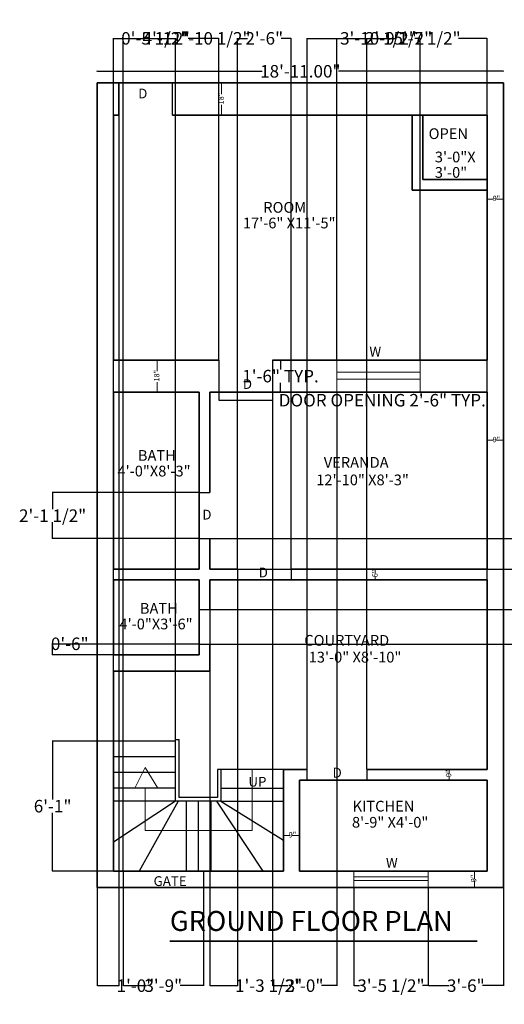
# Model space of a CAD drawing. Units: inches. Extents: x 193743 to 194406, y 400309 to 400860.
# Tile 1 of 2: x 193743 to 194014, y 400309 to 400860. Entities that reach past the tile are written whole.
import ezdxf

# ---------------------------------------------------------------- set-up
doc = ezdxf.new("R2010")
doc.units = ezdxf.units.IN
doc.header["$MEASUREMENT"] = 0
for name, color, linetype, lineweight in [('A-ANNO-DIMS', 2, 'Continuous', 18), ('A-ANNO-SYMB', 7, 'Continuous', 18), ('A-ANNO-TEXT', 7, 'Continuous', 18), ('A-ANNO-TITL', 7, 'Continuous', 35), ('A-AREA-IDEN', 7, 'Continuous', 18), ('A-DOOR', 3, 'Continuous', 25), ('A-FLOR-STRS', 7, 'Continuous', 25), ('A-GLAZ', 4, 'Continuous', 18), ('A-WALL', 7, 'Continuous', 35)]:
    doc.layers.add(name, color=color, linetype=linetype, lineweight=lineweight)
doc.styles.get("Standard").update_dxf_attribs({"font": 'arial.ttf'})
doc.dimstyles.get("Standard").update_dxf_attribs({"dimtxt": 7, "dimasz": 0.18, "dimexe": 0.18, "dimexo": 0.0625, "dimgap": 0.09, "dimtad": 0, "dimtih": 1, "dimtoh": 1, "dimzin": 0, "dimdsep": 46, "dimlunit": 3, "dimtxsty": 'Standard', "dimcen": 0.09, "dimadec": 0, "dimazin": 0, "dimtfac": 1, "dimtofl": 0, "dimtmove": 0, "dimatfit": 3, "dimfxl": 1, "dimtolj": 1, "dimtzin": 0, "dimarcsym": 0})

# ---------------------------------------------------------------- blocks, each defined once
blk = doc.blocks.new('*D1')
at = {"layer": 'A-ANNO-DIMS', "color": 0, "lineweight": -2, "transparency": 16777216}
for p, q in [((193786.7, 400830.65), (193786.7, 400830.94)), ((193786.88, 400830.76), (193878.9, 400830.76)), ((194013.52, 400830.76), (193921.5, 400830.76)), ((194013.7, 400830.65), (194013.7, 400830.94))]:
    blk.add_line(p, q, dxfattribs=at)
at = {"layer": 'A-ANNO-DIMS', "color": 0, "lineweight": 100, "transparency": 16777216}
for points in [[(193786.88, 400830.79), (193786.88, 400830.73), (193786.7, 400830.76)], [(194013.52, 400830.79), (194013.52, 400830.73), (194013.7, 400830.76)]]:
    blk.add_solid(points, dxfattribs=at)
at = {"layer": 'Defpoints', "color": 0, "lineweight": 100, "transparency": 16777216}
for p in [(193786.7, 400830.59), (194013.7, 400830.76), (194013.7, 400830.59)]:
    blk.add_point(p, dxfattribs=at)
at = {"layer": 'A-ANNO-DIMS', "color": 0, "transparency": 16777216, "insert": (193900.2, 400830.76), "char_height": 7, "attachment_point": 5}
blk.add_mtext('\\A1;18\'-11.00"', dxfattribs=at)
blk = doc.blocks.new('SHAFT-RETURN-36X36')
for p, q in [((0, 42), (0, 0)), ((6, 42), (6, 6)), ((6, 6), (42, 6)), ((0, 0), (42, 0))]:
    blk.add_line(p, q)
blk = doc.blocks.new('DOOR-OPENING-30-W18')
for p, q in [((0, 18), (0, 0)), ((29.9, 18), (29.9, 0))]:
    blk.add_line(p, q)
blk = doc.blocks.new('THICKNESS-18-V')
for p, q in [((0, 18), (0, 11.82)), ((0, 5.67), (0, 0))]:
    blk.add_line(p, q)
blk.add_text('18"', height=3, rotation=90).set_placement((1.23, 5.98))
blk = doc.blocks.new('THICKNESS-9-H')
for p, q in [((0, 1.15), (3.54, 1.15)), ((5.14, 1.15), (9, 1.15))]:
    blk.add_line(p, q)
blk.add_text('9"', height=3).set_placement((2.97, 0))
blk = doc.blocks.new('THICKNESS-9-V')
for p, q in [((0.06, 9), (0.06, 5.01)), ((0, 3.6), (0, 0))]:
    blk.add_line(p, q)
blk.add_text('9"', height=3, rotation=90).set_placement((1.05, 2.9))
blk = doc.blocks.new('ROOM-TAG-OPEN-3X3')
for s, p in [('OPEN', (0, 21.67)), ('3\'-0"X', (3.49, 8.63)), ('3\'-0"', (3.46, 0))]:
    blk.add_text(s, height=6).set_placement(p)
blk = doc.blocks.new('*D12')
at = {"layer": 'A-ANNO-DIMS', "color": 0, "lineweight": -2, "transparency": 16777216}
for p, q in [((193854.72, 400651.18), (193854.72, 400646.58)), ((193884.62, 400651.18), (193884.62, 400646.58)), ((193854.9, 400646.76), (193884.44, 400646.76)), ((193884.62, 400646.76), (193884.8, 400646.76))]:
    blk.add_line(p, q, dxfattribs=at)
at = {"layer": 'A-ANNO-DIMS', "color": 0, "lineweight": 100, "transparency": 16777216}
for points in [[(193854.9, 400646.79), (193854.9, 400646.73), (193854.72, 400646.76)], [(193884.44, 400646.79), (193884.44, 400646.73), (193884.62, 400646.76)]]:
    blk.add_solid(points, dxfattribs=at)
at = {"layer": 'Defpoints', "color": 0, "lineweight": 100, "transparency": 16777216}
for p in [(193854.72, 400651.24), (193884.62, 400651.24), (193884.62, 400646.76)]:
    blk.add_point(p, dxfattribs=at)
at = {"layer": 'A-ANNO-DIMS', "color": 0, "transparency": 16777216, "insert": (193945.99, 400646.76), "char_height": 7, "attachment_point": 5}
blk.add_mtext('\\A1;DOOR OPENING 2\'-6" TYP.', dxfattribs=at)
blk = doc.blocks.new('*D13')
at = {"layer": 'A-ANNO-DIMS', "color": 0, "lineweight": -2, "transparency": 16777216}
for p, q in [((193884.68, 400669.24), (193889.29, 400669.24)), ((193889.11, 400669.06), (193889.11, 400663.9)), ((193889.11, 400651.42), (193889.11, 400656.58)), ((193884.68, 400651.24), (193889.29, 400651.24))]:
    blk.add_line(p, q, dxfattribs=at)
at = {"layer": 'A-ANNO-DIMS', "color": 0, "lineweight": 100, "transparency": 16777216}
for points in [[(193889.08, 400669.06), (193889.14, 400669.06), (193889.11, 400669.24)], [(193889.08, 400651.42), (193889.14, 400651.42), (193889.11, 400651.24)]]:
    blk.add_solid(points, dxfattribs=at)
at = {"layer": 'Defpoints', "color": 0, "lineweight": 100, "transparency": 16777216}
for p in [(193884.62, 400669.24), (193889.11, 400669.24), (193884.62, 400651.24)]:
    blk.add_point(p, dxfattribs=at)
at = {"layer": 'A-ANNO-DIMS', "color": 0, "transparency": 16777216, "insert": (193889.11, 400660.24), "char_height": 7, "attachment_point": 5}
blk.add_mtext('\\A1;1\'-6" TYP.', dxfattribs=at)
blk = doc.blocks.new('*D18')
at = {"layer": 'A-ANNO-DIMS', "color": 0, "lineweight": -2, "transparency": 16777216}
for p, q in [((193795.7, 400383.3), (193795.7, 400849.37)), ((193795.88, 400849.19), (193800.94, 400849.19)), ((193801.12, 400383.3), (193801.12, 400849.37)), ((193801.12, 400849.19), (193801.3, 400849.19))]:
    blk.add_line(p, q, dxfattribs=at)
at = {"layer": 'A-ANNO-DIMS', "color": 0, "lineweight": 100, "transparency": 16777216}
for points in [[(193795.88, 400849.22), (193795.88, 400849.16), (193795.7, 400849.19)], [(193800.94, 400849.22), (193800.94, 400849.16), (193801.12, 400849.19)]]:
    blk.add_solid(points, dxfattribs=at)
at = {"layer": 'Defpoints', "color": 0, "lineweight": 100, "transparency": 16777216}
for p in [(193801.12, 400849.19), (193795.7, 400383.24), (193801.12, 400383.24)]:
    blk.add_point(p, dxfattribs=at)
at = {"layer": 'A-ANNO-DIMS', "color": 0, "transparency": 16777216, "insert": (193818.85, 400849.19), "char_height": 7, "attachment_point": 5}
blk.add_mtext('\\A1;0\'-5 1/2"', dxfattribs=at)
blk = doc.blocks.new('*D19')
at = {"layer": 'A-ANNO-DIMS', "color": 0, "lineweight": -2, "transparency": 16777216}
for p, q in [((193801.12, 400374.18), (193801.12, 400319.09)), ((193846.06, 400374.18), (193846.06, 400319.09)), ((193801.3, 400319.27), (193814.2, 400319.27)), ((193845.88, 400319.27), (193832.98, 400319.27))]:
    blk.add_line(p, q, dxfattribs=at)
at = {"layer": 'A-ANNO-DIMS', "color": 0, "lineweight": 100, "transparency": 16777216}
for points in [[(193801.3, 400319.3), (193801.3, 400319.24), (193801.12, 400319.27)], [(193845.88, 400319.3), (193845.88, 400319.24), (193846.06, 400319.27)]]:
    blk.add_solid(points, dxfattribs=at)
at = {"layer": 'Defpoints', "color": 0, "lineweight": 100, "transparency": 16777216}
for p in [(193801.12, 400374.24), (193846.06, 400374.24), (193846.06, 400319.27)]:
    blk.add_point(p, dxfattribs=at)
at = {"layer": 'A-ANNO-DIMS', "color": 0, "transparency": 16777216, "insert": (193823.59, 400319.27), "char_height": 7, "attachment_point": 5}
blk.add_mtext('\\A1;3\'-9"', dxfattribs=at)
blk = doc.blocks.new('*D20')
at = {"layer": 'A-ANNO-DIMS', "color": 0, "lineweight": -2, "transparency": 16777216}
for p, q in [((193930.04, 400374.18), (193930.04, 400319.09)), ((193971.71, 400374.18), (193971.71, 400319.09)), ((193930.22, 400319.27), (193933.33, 400319.27)), ((193971.53, 400319.27), (193968.42, 400319.27))]:
    blk.add_line(p, q, dxfattribs=at)
at = {"layer": 'A-ANNO-DIMS', "color": 0, "lineweight": 100, "transparency": 16777216}
for points in [[(193930.22, 400319.3), (193930.22, 400319.24), (193930.04, 400319.27)], [(193971.53, 400319.3), (193971.53, 400319.24), (193971.71, 400319.27)]]:
    blk.add_solid(points, dxfattribs=at)
at = {"layer": 'Defpoints', "color": 0, "lineweight": 100, "transparency": 16777216}
for p in [(193930.04, 400374.24), (193971.71, 400374.24), (193971.71, 400319.27)]:
    blk.add_point(p, dxfattribs=at)
at = {"layer": 'A-ANNO-DIMS', "color": 0, "transparency": 16777216, "insert": (193950.87, 400319.27), "char_height": 7, "attachment_point": 5}
blk.add_mtext('\\A1;3\'-5 1/2"', dxfattribs=at)
blk = doc.blocks.new('*D21')
at = {"layer": 'A-ANNO-DIMS', "color": 0, "lineweight": -2, "transparency": 16777216}
for p, q in [((193971.71, 400374.18), (193971.71, 400319.09)), ((194013.7, 400374.18), (194013.7, 400319.09)), ((193971.89, 400319.27), (193983.31, 400319.27)), ((194013.52, 400319.27), (194002.09, 400319.27))]:
    blk.add_line(p, q, dxfattribs=at)
at = {"layer": 'A-ANNO-DIMS', "color": 0, "lineweight": 100, "transparency": 16777216}
for points in [[(193971.89, 400319.3), (193971.89, 400319.24), (193971.71, 400319.27)], [(194013.52, 400319.3), (194013.52, 400319.24), (194013.7, 400319.27)]]:
    blk.add_solid(points, dxfattribs=at)
at = {"layer": 'Defpoints', "color": 0, "lineweight": 100, "transparency": 16777216}
for p in [(193971.71, 400374.24), (194013.7, 400374.24), (194013.7, 400319.27)]:
    blk.add_point(p, dxfattribs=at)
at = {"layer": 'A-ANNO-DIMS', "color": 0, "transparency": 16777216, "insert": (193992.7, 400319.27), "char_height": 7, "attachment_point": 5}
blk.add_mtext('\\A1;3\'-6"', dxfattribs=at)
blk = doc.blocks.new('*D22')
at = {"layer": 'A-ANNO-DIMS', "color": 0, "lineweight": -2, "transparency": 16777216}
for p, q in [((193786.7, 400824.18), (193786.7, 400319.09)), ((193798.79, 400824.18), (193798.79, 400319.09)), ((193786.88, 400319.27), (193798.61, 400319.27)), ((193798.79, 400319.27), (193798.97, 400319.27))]:
    blk.add_line(p, q, dxfattribs=at)
at = {"layer": 'A-ANNO-DIMS', "color": 0, "lineweight": 100, "transparency": 16777216}
for points in [[(193786.88, 400319.3), (193786.88, 400319.24), (193786.7, 400319.27)], [(193798.61, 400319.3), (193798.61, 400319.24), (193798.79, 400319.27)]]:
    blk.add_solid(points, dxfattribs=at)
at = {"layer": 'Defpoints', "color": 0, "lineweight": 100, "transparency": 16777216}
for p in [(193786.7, 400824.24), (193798.79, 400824.24), (193798.79, 400319.27)]:
    blk.add_point(p, dxfattribs=at)
at = {"layer": 'A-ANNO-DIMS', "color": 0, "transparency": 16777216, "insert": (193808.03, 400319.27), "char_height": 7, "attachment_point": 5}
blk.add_mtext('\\A1;1\'-0"', dxfattribs=at)
blk = doc.blocks.new('*D23')
at = {"layer": 'A-ANNO-DIMS', "color": 0, "lineweight": -2, "transparency": 16777216}
for p, q in [((193795.7, 400669.3), (193795.7, 400849.37)), ((193795.88, 400849.19), (193812.95, 400849.19)), ((193854.54, 400849.19), (193837.46, 400849.19)), ((193854.72, 400669.3), (193854.72, 400849.37))]:
    blk.add_line(p, q, dxfattribs=at)
at = {"layer": 'A-ANNO-DIMS', "color": 0, "lineweight": 100, "transparency": 16777216}
for points in [[(193795.88, 400849.22), (193795.88, 400849.16), (193795.7, 400849.19)], [(193854.54, 400849.22), (193854.54, 400849.16), (193854.72, 400849.19)]]:
    blk.add_solid(points, dxfattribs=at)
at = {"layer": 'Defpoints', "color": 0, "lineweight": 100, "transparency": 16777216}
for p in [(193854.72, 400849.19), (193795.7, 400669.24), (193854.72, 400669.24)]:
    blk.add_point(p, dxfattribs=at)
at = {"layer": 'A-ANNO-DIMS', "color": 0, "transparency": 16777216, "insert": (193825.21, 400849.19), "char_height": 7, "attachment_point": 5}
blk.add_mtext('\\A1;4\'-11"', dxfattribs=at)
blk = doc.blocks.new('*D24')
at = {"layer": 'A-ANNO-DIMS', "color": 0, "lineweight": -2, "transparency": 16777216}
for p, q in [((193920.54, 400669.3), (193920.54, 400849.37)), ((193920.72, 400849.19), (193923.58, 400849.19)), ((193966.98, 400849.19), (193964.12, 400849.19)), ((193967.16, 400669.3), (193967.16, 400849.37))]:
    blk.add_line(p, q, dxfattribs=at)
at = {"layer": 'A-ANNO-DIMS', "color": 0, "lineweight": 100, "transparency": 16777216}
for points in [[(193920.72, 400849.22), (193920.72, 400849.16), (193920.54, 400849.19)], [(193966.98, 400849.22), (193966.98, 400849.16), (193967.16, 400849.19)]]:
    blk.add_solid(points, dxfattribs=at)
at = {"layer": 'Defpoints', "color": 0, "lineweight": 100, "transparency": 16777216}
for p in [(193967.16, 400849.19), (193920.54, 400669.24), (193967.16, 400669.24)]:
    blk.add_point(p, dxfattribs=at)
at = {"layer": 'A-ANNO-DIMS', "color": 0, "transparency": 16777216, "insert": (193943.85, 400849.19), "char_height": 7, "attachment_point": 5}
blk.add_mtext('\\A1;3\'-10 1/2"', dxfattribs=at)
blk = doc.blocks.new('*D25')
at = {"layer": 'A-ANNO-DIMS', "color": 0, "lineweight": -2, "transparency": 16777216}
for p, q in [((193884.62, 400651.18), (193884.62, 400319.09)), ((193920.54, 400651.18), (193920.54, 400319.09)), ((193884.8, 400319.27), (193893.19, 400319.27)), ((193920.36, 400319.27), (193911.97, 400319.27))]:
    blk.add_line(p, q, dxfattribs=at)
at = {"layer": 'A-ANNO-DIMS', "color": 0, "lineweight": 100, "transparency": 16777216}
for points in [[(193884.8, 400319.3), (193884.8, 400319.24), (193884.62, 400319.27)], [(193920.36, 400319.3), (193920.36, 400319.24), (193920.54, 400319.27)]]:
    blk.add_solid(points, dxfattribs=at)
at = {"layer": 'Defpoints', "color": 0, "lineweight": 100, "transparency": 16777216}
for p in [(193884.62, 400651.24), (193920.54, 400651.24), (193920.54, 400319.27)]:
    blk.add_point(p, dxfattribs=at)
at = {"layer": 'A-ANNO-DIMS', "color": 0, "transparency": 16777216, "insert": (193902.58, 400319.27), "char_height": 7, "attachment_point": 5}
blk.add_mtext('\\A1;3\'-0"', dxfattribs=at)
blk = doc.blocks.new('*D26')
at = {"layer": 'A-ANNO-DIMS', "color": 0, "lineweight": -2, "transparency": 16777216}
for p, q in [((193849.7, 400546.18), (193849.7, 400319.09)), ((193865.1, 400546.18), (193865.1, 400319.09)), ((193849.88, 400319.27), (193864.92, 400319.27)), ((193865.1, 400319.27), (193865.28, 400319.27))]:
    blk.add_line(p, q, dxfattribs=at)
at = {"layer": 'A-ANNO-DIMS', "color": 0, "lineweight": 100, "transparency": 16777216}
for points in [[(193849.88, 400319.3), (193849.88, 400319.24), (193849.7, 400319.27)], [(193864.92, 400319.3), (193864.92, 400319.24), (193865.1, 400319.27)]]:
    blk.add_solid(points, dxfattribs=at)
at = {"layer": 'Defpoints', "color": 0, "lineweight": 100, "transparency": 16777216}
for p in [(193849.7, 400546.24), (193865.1, 400546.24), (193865.1, 400319.27)]:
    blk.add_point(p, dxfattribs=at)
at = {"layer": 'A-ANNO-DIMS', "color": 0, "transparency": 16777216, "insert": (193882.5, 400319.27), "char_height": 7, "attachment_point": 5}
blk.add_mtext('\\A1;1\'-3 1/2"', dxfattribs=at)
blk = doc.blocks.new('*D27')
at = {"layer": 'A-ANNO-DIMS', "color": 0, "lineweight": -2, "transparency": 16777216}
for p, q in [((193865.1, 400552.3), (193865.1, 400849.37)), ((193865.28, 400849.19), (193870.6, 400849.19)), ((193894.82, 400849.19), (193889.51, 400849.19)), ((193895, 400552.3), (193895, 400849.37))]:
    blk.add_line(p, q, dxfattribs=at)
at = {"layer": 'A-ANNO-DIMS', "color": 0, "lineweight": 100, "transparency": 16777216}
for points in [[(193865.28, 400849.22), (193865.28, 400849.16), (193865.1, 400849.19)], [(193894.82, 400849.22), (193894.82, 400849.16), (193895, 400849.19)]]:
    blk.add_solid(points, dxfattribs=at)
at = {"layer": 'Defpoints', "color": 0, "lineweight": 100, "transparency": 16777216}
for p in [(193895, 400849.19), (193865.1, 400552.24), (193895, 400552.24)]:
    blk.add_point(p, dxfattribs=at)
at = {"layer": 'A-ANNO-DIMS', "color": 0, "transparency": 16777216, "insert": (193880.05, 400849.19), "char_height": 7, "attachment_point": 5}
blk.add_mtext('\\A1;2\'-6"', dxfattribs=at)
blk = doc.blocks.new('*D28')
at = {"layer": 'A-ANNO-DIMS', "color": 0, "lineweight": -2, "transparency": 16777216}
for p, q in [((193849.76, 400569.32), (194038.83, 400569.32)), ((194038.65, 400569.14), (194038.65, 400564.44)), ((194038.65, 400552.42), (194038.65, 400557.12)), ((193849.76, 400552.24), (194038.83, 400552.24))]:
    blk.add_line(p, q, dxfattribs=at)
at = {"layer": 'A-ANNO-DIMS', "color": 0, "lineweight": 100, "transparency": 16777216}
for points in [[(194038.62, 400569.14), (194038.68, 400569.14), (194038.65, 400569.32)], [(194038.62, 400552.42), (194038.68, 400552.42), (194038.65, 400552.24)]]:
    blk.add_solid(points, dxfattribs=at)
at = {"layer": 'Defpoints', "color": 0, "lineweight": 100, "transparency": 16777216}
for p in [(193849.7, 400569.32), (194038.65, 400569.32), (193849.7, 400552.24)]:
    blk.add_point(p, dxfattribs=at)
at = {"layer": 'A-ANNO-DIMS', "color": 0, "transparency": 16777216, "insert": (194038.65, 400560.78), "char_height": 7, "attachment_point": 5}
blk.add_mtext('\\A1;1\'-5"', dxfattribs=at)
blk = doc.blocks.new('*D29')
at = {"layer": 'A-ANNO-DIMS', "color": 0, "lineweight": -2, "transparency": 16777216}
for p, q in [((193843.63, 400595.05), (193761.57, 400595.05)), ((193761.75, 400594.87), (193761.75, 400585.89)), ((193761.75, 400569.5), (193761.75, 400578.48)), ((193843.63, 400569.32), (193761.57, 400569.32))]:
    blk.add_line(p, q, dxfattribs=at)
at = {"layer": 'A-ANNO-DIMS', "color": 0, "lineweight": 100, "transparency": 16777216}
for points in [[(193761.72, 400594.87), (193761.78, 400594.87), (193761.75, 400595.05)], [(193761.72, 400569.5), (193761.78, 400569.5), (193761.75, 400569.32)]]:
    blk.add_solid(points, dxfattribs=at)
at = {"layer": 'Defpoints', "color": 0, "lineweight": 100, "transparency": 16777216}
for p in [(193761.75, 400595.05), (193843.7, 400595.05), (193843.7, 400569.32)]:
    blk.add_point(p, dxfattribs=at)
at = {"layer": 'A-ANNO-DIMS', "color": 0, "transparency": 16777216, "insert": (193761.75, 400582.19), "char_height": 7, "attachment_point": 5}
blk.add_mtext('\\A1;2\'-1 1/2"', dxfattribs=at)
blk = doc.blocks.new('*D30')
at = {"layer": 'A-ANNO-DIMS', "color": 0, "lineweight": -2, "transparency": 16777216}
for p, q in [((193843.63, 400510.32), (193761.57, 400510.32)), ((193761.75, 400510.32), (193761.75, 400510.5)), ((193761.75, 400510.5), (193761.93, 400510.5)), ((193761.75, 400504.42), (193761.75, 400510.14)), ((193843.63, 400504.24), (193761.57, 400504.24))]:
    blk.add_line(p, q, dxfattribs=at)
at = {"layer": 'A-ANNO-DIMS', "color": 0, "lineweight": 100, "transparency": 16777216}
for points in [[(193761.72, 400510.14), (193761.78, 400510.14), (193761.75, 400510.32)], [(193761.72, 400504.42), (193761.78, 400504.42), (193761.75, 400504.24)]]:
    blk.add_solid(points, dxfattribs=at)
at = {"layer": 'Defpoints', "color": 0, "lineweight": 100, "transparency": 16777216}
for p in [(193761.75, 400510.32), (193843.7, 400510.32), (193843.7, 400504.24)]:
    blk.add_point(p, dxfattribs=at)
at = {"layer": 'A-ANNO-DIMS', "color": 0, "transparency": 16777216, "insert": (193771.32, 400510.5), "char_height": 7, "attachment_point": 5}
blk.add_mtext('\\A1;0\'-6"', dxfattribs=at)
blk = doc.blocks.new('*D31')
at = {"layer": 'A-ANNO-DIMS', "color": 0, "lineweight": -2, "transparency": 16777216}
for p, q in [((193849.76, 400529.76), (194038.83, 400529.76)), ((194038.65, 400529.58), (194038.65, 400523.75)), ((194038.65, 400510.5), (194038.65, 400516.33)), ((193849.76, 400510.32), (194038.83, 400510.32))]:
    blk.add_line(p, q, dxfattribs=at)
at = {"layer": 'A-ANNO-DIMS', "color": 0, "lineweight": 100, "transparency": 16777216}
for points in [[(194038.62, 400529.58), (194038.68, 400529.58), (194038.65, 400529.76)], [(194038.62, 400510.5), (194038.68, 400510.5), (194038.65, 400510.32)]]:
    blk.add_solid(points, dxfattribs=at)
at = {"layer": 'Defpoints', "color": 0, "lineweight": 100, "transparency": 16777216}
for p in [(193849.7, 400529.76), (193849.7, 400510.32), (194038.65, 400510.32)]:
    blk.add_point(p, dxfattribs=at)
at = {"layer": 'A-ANNO-DIMS', "color": 0, "transparency": 16777216, "insert": (194038.65, 400520.04), "char_height": 7, "attachment_point": 5}
blk.add_mtext('\\A1;1\'-7 1/2"', dxfattribs=at)
blk = doc.blocks.new('*D32')
at = {"layer": 'A-ANNO-DIMS', "color": 0, "lineweight": -2, "transparency": 16777216}
for p, q in [((193904.1, 400440.3), (193904.1, 400849.37)), ((193904.28, 400849.19), (193937.18, 400849.19)), ((193937.36, 400440.3), (193937.36, 400849.37)), ((193937.36, 400849.19), (193937.54, 400849.19))]:
    blk.add_line(p, q, dxfattribs=at)
at = {"layer": 'A-ANNO-DIMS', "color": 0, "lineweight": 100, "transparency": 16777216}
for points in [[(193904.28, 400849.22), (193904.28, 400849.16), (193904.1, 400849.19)], [(193937.18, 400849.22), (193937.18, 400849.16), (193937.36, 400849.19)]]:
    blk.add_solid(points, dxfattribs=at)
at = {"layer": 'Defpoints', "color": 0, "lineweight": 100, "transparency": 16777216}
for p in [(193937.36, 400849.19), (193904.1, 400440.24), (193937.36, 400440.24)]:
    blk.add_point(p, dxfattribs=at)
at = {"layer": 'A-ANNO-DIMS', "color": 0, "transparency": 16777216, "insert": (193955.15, 400849.19), "char_height": 7, "attachment_point": 5}
blk.add_mtext('\\A1;2\'-9 1/2"', dxfattribs=at)
blk = doc.blocks.new('*D33')
at = {"layer": 'A-ANNO-DIMS', "color": 0, "lineweight": -2, "transparency": 16777216}
for p, q in [((193937.36, 400440.3), (193937.36, 400849.37)), ((193937.54, 400849.19), (193953.48, 400849.19)), ((194004.52, 400849.19), (193988.58, 400849.19)), ((194004.7, 400440.3), (194004.7, 400849.37))]:
    blk.add_line(p, q, dxfattribs=at)
at = {"layer": 'A-ANNO-DIMS', "color": 0, "lineweight": 100, "transparency": 16777216}
for points in [[(193937.54, 400849.22), (193937.54, 400849.16), (193937.36, 400849.19)], [(194004.52, 400849.22), (194004.52, 400849.16), (194004.7, 400849.19)]]:
    blk.add_solid(points, dxfattribs=at)
at = {"layer": 'Defpoints', "color": 0, "lineweight": 100, "transparency": 16777216}
for p in [(194004.7, 400849.19), (193937.36, 400440.24), (194004.7, 400440.24)]:
    blk.add_point(p, dxfattribs=at)
at = {"layer": 'A-ANNO-DIMS', "color": 0, "transparency": 16777216, "insert": (193971.03, 400849.19), "char_height": 7, "attachment_point": 5}
blk.add_mtext('\\A1;5\'-7 1/2"', dxfattribs=at)
blk = doc.blocks.new('*D34')
at = {"layer": 'A-ANNO-DIMS', "color": 0, "lineweight": -2, "transparency": 16777216}
for p, q in [((193795.7, 400456.18), (193795.7, 400849.37)), ((193795.88, 400849.19), (193830.26, 400849.19)), ((193830.44, 400456.18), (193830.44, 400849.37)), ((193830.44, 400849.19), (193830.62, 400849.19))]:
    blk.add_line(p, q, dxfattribs=at)
at = {"layer": 'A-ANNO-DIMS', "color": 0, "lineweight": 100, "transparency": 16777216}
for points in [[(193795.88, 400849.22), (193795.88, 400849.16), (193795.7, 400849.19)], [(193830.26, 400849.22), (193830.26, 400849.16), (193830.44, 400849.19)]]:
    blk.add_solid(points, dxfattribs=at)
at = {"layer": 'Defpoints', "color": 0, "lineweight": 100, "transparency": 16777216}
for p in [(193830.44, 400849.19), (193795.7, 400456.12), (193830.44, 400456.12)]:
    blk.add_point(p, dxfattribs=at)
at = {"layer": 'A-ANNO-DIMS', "color": 0, "transparency": 16777216, "insert": (193850.94, 400849.19), "char_height": 7, "attachment_point": 5}
blk.add_mtext('\\A1;2\'-10 1/2"', dxfattribs=at)
blk = doc.blocks.new('*D35')
at = {"layer": 'A-ANNO-DIMS', "color": 0, "lineweight": -2, "transparency": 16777216}
for p, q in [((193795.63, 400456.12), (193761.57, 400456.12)), ((193761.75, 400455.94), (193761.75, 400423.35)), ((193761.75, 400383.42), (193761.75, 400416.02)), ((193795.63, 400383.24), (193761.57, 400383.24))]:
    blk.add_line(p, q, dxfattribs=at)
at = {"layer": 'A-ANNO-DIMS', "color": 0, "lineweight": 100, "transparency": 16777216}
for points in [[(193761.72, 400455.94), (193761.78, 400455.94), (193761.75, 400456.12)], [(193761.72, 400383.42), (193761.78, 400383.42), (193761.75, 400383.24)]]:
    blk.add_solid(points, dxfattribs=at)
at = {"layer": 'Defpoints', "color": 0, "lineweight": 100, "transparency": 16777216}
for p in [(193761.75, 400456.12), (193795.7, 400456.12), (193795.7, 400383.24)]:
    blk.add_point(p, dxfattribs=at)
at = {"layer": 'A-ANNO-DIMS', "color": 0, "transparency": 16777216, "insert": (193761.75, 400419.68), "char_height": 7, "attachment_point": 5}
blk.add_mtext('\\A1;6\'-1"', dxfattribs=at)

msp = doc.modelspace()

# ---------------------------------------------------------------- linework, layer by layer
at = {"layer": 'A-ANNO-DIMS'}
for p, q in [((193942.101, 400552.24), (193942.101, 400552.24)), ((193942.101, 400552.24), (193942.101, 400549.774)), ((193942.101, 400547.811), (193942.101, 400546.24)), ((193983.342, 400438.066), (193983.342, 400440.24)), ((193983.342, 400436.447), (193983.342, 400434.24))]:
    msp.add_line(p, q, dxfattribs=at)
at = {"layer": 'A-ANNO-SYMB'}
for p, q in [((193807.697, 400429.723), (193813.541, 400441.344)), ((193813.541, 400441.344), (193820.557, 400429.723)), ((193873.253, 400440.24), (193873.253, 400406.096)), ((193813.541, 400429.723), (193807.697, 400429.723)), ((193813.541, 400406.096), (193813.541, 400429.723)), ((193873.253, 400406.096), (193813.541, 400406.096))]:
    msp.add_line(p, q, dxfattribs=at)
at = {"layer": 'A-ANNO-TITL'}
msp.add_line((193827.283, 400344.223), (193999.094, 400344.223), dxfattribs=at)
at = {"layer": 'A-DOOR'}
for p, q in [((193843.697, 400595.052), (193849.697, 400595.052)), ((193843.697, 400569.318), (193849.697, 400569.318)), ((193865.104, 400552.24), (193865.104, 400546.24)), ((193895.003, 400552.24), (193895.003, 400546.24)), ((193843.697, 400529.763), (193849.697, 400529.763)), ((193843.697, 400510.321), (193849.697, 400510.321)), ((193904.104, 400434.24), (193904.104, 400440.24)), ((193937.364, 400440.24), (193937.364, 400434.24)), ((193801.119, 400383.24), (193801.119, 400374.24)), ((193846.055, 400383.24), (193846.055, 400374.24))]:
    msp.add_line(p, q, dxfattribs=at)
at = {"layer": 'A-FLOR-STRS'}
for p, q in [((193830.436, 400456.122), (193795.697, 400456.122)), ((193830.436, 400422.546), (193830.436, 400457.001)), ((193830.436, 400457.001), (193832.436, 400457.001)), ((193832.436, 400424.546), (193832.436, 400457.001)), ((193830.436, 400447.322), (193795.697, 400447.322)), ((193830.436, 400438.523), (193795.697, 400438.523)), ((193890.697, 400440.24), (193853.809, 400440.24)), ((193853.809, 400440.24), (193853.809, 400424.546)), ((193855.809, 400440.24), (193855.809, 400422.546)), ((193830.436, 400429.723), (193795.697, 400429.723)), ((193855.809, 400429.723), (193890.697, 400429.723)), ((193830.436, 400422.546), (193795.697, 400422.546)), ((193830.436, 400422.546), (193795.697, 400399.547)), ((193831.952, 400422.546), (193810.193, 400383.24)), ((193855.809, 400422.546), (193830.436, 400422.546)), ((193853.809, 400424.546), (193832.436, 400424.546)), ((193836.323, 400422.546), (193836.323, 400383.24)), ((193843.123, 400422.546), (193843.123, 400383.24)), ((193850.233, 400422.546), (193850.233, 400383.24)), ((193853.412, 400422.546), (193879.244, 400383.24)), ((193855.809, 400422.546), (193890.697, 400400.738)), ((193855.809, 400422.546), (193890.697, 400422.546))]:
    msp.add_line(p, q, dxfattribs=at)
at = {"layer": 'A-GLAZ'}
for p, q in [((193920.537, 400669.24), (193920.537, 400651.24)), ((193967.161, 400669.24), (193967.161, 400669.24)), ((193967.161, 400669.24), (193967.161, 400651.24)), ((193920.537, 400662.472), (193967.161, 400662.472)), ((193920.537, 400658.511), (193967.161, 400658.511)), ((193930.039, 400383.24), (193930.039, 400374.24)), ((193971.709, 400383.24), (193971.709, 400374.24)), ((193971.709, 400380.221), (193930.039, 400380.221)), ((193930.039, 400380.221), (193930.039, 400378.07)), ((193930.039, 400378.07), (193971.709, 400378.07)), ((193971.709, 400374.24), (193971.709, 400380.221))]:
    msp.add_line(p, q, dxfattribs=at)
at = {"layer": 'A-WALL'}
for p, q in [((193786.697, 400824.24), (194013.697, 400824.24)), ((193786.697, 400374.24), (193786.697, 400824.24)), ((194013.697, 400824.24), (194013.697, 400374.24)), ((193795.697, 400806.24), (193798.787, 400806.24)), ((193795.697, 400669.24), (193795.697, 400806.24)), ((193828.686, 400806.24), (194004.697, 400806.24)), ((194004.697, 400806.24), (194004.697, 400669.24)), ((193795.697, 400669.24), (193854.721, 400669.24)), ((193884.621, 400669.24), (194004.697, 400669.24)), ((193795.697, 400651.24), (193843.697, 400651.24)), ((193795.697, 400552.24), (193795.697, 400651.24)), ((193843.697, 400552.24), (193843.697, 400651.24)), ((193843.697, 400552.24), (193843.697, 400651.24)), ((193849.697, 400651.24), (194004.697, 400651.24)), ((193849.697, 400595.052), (193849.697, 400651.24)), ((193849.697, 400595.052), (193849.697, 400651.24)), ((194004.697, 400651.24), (194004.697, 400552.24)), ((193849.697, 400552.24), (193849.697, 400569.318)), ((193849.697, 400552.24), (193849.697, 400569.318)), ((193795.697, 400552.24), (193843.697, 400552.24)), ((193849.697, 400552.24), (193865.104, 400552.24)), ((193895.003, 400552.24), (194004.697, 400552.24)), ((193795.697, 400546.24), (193843.697, 400546.24)), ((193795.697, 400504.24), (193795.697, 400546.24)), ((193843.697, 400504.24), (193843.697, 400546.24)), ((193849.697, 400546.24), (194004.697, 400546.24)), ((193849.697, 400529.763), (193849.697, 400546.24)), ((194004.697, 400546.24), (194004.697, 400440.24)), ((193849.697, 400495.24), (193849.697, 400510.321)), ((193795.697, 400504.24), (193843.697, 400504.24)), ((193795.697, 400383.24), (193795.697, 400495.24)), ((193795.697, 400495.24), (193849.697, 400495.24)), ((193890.697, 400440.24), (193904.104, 400440.24)), ((193890.697, 400440.24), (193890.697, 400383.24)), ((193937.364, 400440.24), (194004.697, 400440.24)), ((193899.697, 400434.24), (194004.697, 400434.24)), ((193899.697, 400434.24), (193899.697, 400383.24)), ((194004.697, 400434.24), (194004.697, 400383.24)), ((193890.697, 400383.24), (193795.697, 400383.24)), ((194004.697, 400383.24), (193899.697, 400383.24)), ((194013.697, 400374.24), (193786.697, 400374.24))]:
    msp.add_line(p, q, dxfattribs=at)

# ---------------------------------------------------------------- block references
at = {"layer": 'A-ANNO-DIMS'}
for name, p in [('THICKNESS-18-V', (193856.126, 400806.24)), ('THICKNESS-9-H', (194004.697, 400758.15)), ('THICKNESS-18-V', (193820.16, 400651.24)), ('THICKNESS-9-H', (194004.697, 400623.235)), ('THICKNESS-9-H', (193890.697, 400402.176)), ('THICKNESS-9-V', (193997.486, 400374.24))]:
    msp.add_blockref(name, p, dxfattribs=at)
at = {"layer": 'A-AREA-IDEN'}
msp.add_blockref('ROOM-TAG-OPEN-3X3', (193971.914, 400771.193), dxfattribs=at)
at = {"layer": 'A-DOOR', "rotation": 180}
msp.add_blockref('DOOR-OPENING-30-W18', (193828.686, 400824.24), dxfattribs=at)
at = {"layer": 'A-DOOR'}
msp.add_blockref('DOOR-OPENING-30-W18', (193854.721, 400651.24), dxfattribs=at)
at = {"layer": 'A-WALL'}
msp.add_blockref('SHAFT-RETURN-36X36', (193962.697, 400764.24), dxfattribs=at)

# ---------------------------------------------------------------- texts
at = {"layer": 'A-ANNO-DIMS'}
for s, p in [('6"', (193943.429, 400547.687)), ('9"', (193984.564, 400435.963))]:
    msp.add_text(s, height=3, rotation=90, dxfattribs=at).set_placement(p)
at = {"layer": 'A-ANNO-TEXT'}
for s, height, p in [('D', 5.457, (193809.574, 400815.611)), ('W', 5.457, (193938.812, 400671.199)), ('D', 5.457, (193868.075, 400653.075)), ('D', 5.457, (193845.402, 400580.028)), ('D', 5.457, (193876.937, 400547.663)), ('D', 5.457, (193918.227, 400435.668)), ('UP', 5.4573, (193871.167, 400430.612)), ('W', 5.457, (193948.064, 400385.214)), ('GATE', 5.4573, (193818.175, 400375.006))]:
    msp.add_text(s, height=height, dxfattribs=at).set_placement(p)
at = {"layer": 'A-ANNO-TITL'}
msp.add_text('GROUND FLOOR PLAN', height=11.181, dxfattribs=at).set_placement((193827.283, 400349.87))
at = {"layer": 'A-AREA-IDEN'}
for s, p in [('ROOM', (193879.489, 400751.636)), ('17\'-6" X11\'-5"', (193868.088, 400742.895)), ('BATH', (193809.391, 400612.864)), ('VERANDA', (193913.305, 400608.974)), ('4\'-0"X8\'-3"', (193797.99, 400604.123)), ('12\'-10" X8\'-3"', (193909.091, 400599.189)), ('BATH', (193810.51, 400527.325)), ('4\'-0"X3\'-6"', (193799.109, 400518.584)), ('COURTYARD', (193902.416, 400509.44)), ('13\'-0" X8\'-10"', (193904.895, 400500.045)), ('KITCHEN', (193929.414, 400416.66)), ('8\'-9" X4\'-0"', (193929.055, 400407.656))]:
    msp.add_text(s, height=6, dxfattribs=at).set_placement(p)

# ---------------------------------------------------------------- dimensions: what is measured, and where the dimension line sits
at = {"layer": 'A-ANNO-DIMS'}
for base, p1, p2, override, picture, middle in [((193801.119, 400849.19), (193795.697, 400383.24), (193801.119, 400383.24), {"dimdec": 1, "dimlfac": 1, "dimrnd": 0, "dimzin": 1, "dimdsep": 46, "dimlunit": 4, "dimfrac": 2}, '*D18', (193818.849, 400849.19)), ((193830.436, 400849.19), (193795.697, 400456.122), (193830.436, 400456.122), {"dimdec": 1, "dimlfac": 1, "dimrnd": 0, "dimzin": 1, "dimdsep": 46, "dimlunit": 4, "dimfrac": 2}, '*D34', (193850.944, 400849.19)), ((193937.364, 400849.19), (193904.104, 400440.24), (193937.364, 400440.24), {"dimdec": 1, "dimlfac": 1, "dimrnd": 0, "dimzin": 1, "dimdsep": 46, "dimlunit": 4, "dimfrac": 2}, '*D32', (193955.153, 400849.19)), ((193967.161, 400849.19), (193920.537, 400669.24), (193967.161, 400669.24), {"dimdec": 1, "dimlfac": 1, "dimrnd": 0, "dimzin": 1, "dimdsep": 46, "dimlunit": 4, "dimfrac": 2}, '*D24', (193943.849, 400849.19)), ((194004.697, 400849.19), (193937.364, 400440.24), (194004.697, 400440.24), {"dimdec": 1, "dimlfac": 1, "dimrnd": 0, "dimzin": 1, "dimdsep": 46, "dimlunit": 4, "dimfrac": 2}, '*D33', (193971.03, 400849.19)), ((193854.721, 400849.19), (193795.697, 400669.24), (193854.721, 400669.24), {"dimdec": 1, "dimlfac": 1, "dimrnd": 0, "dimzin": 1, "dimdsep": 46, "dimlunit": 4, "dimfrac": 2}, '*D23', (193825.209, 400849.19)), ((193895.003, 400849.19), (193865.104, 400552.24), (193895.003, 400552.24), {"dimdec": 1, "dimlfac": 1, "dimrnd": 0, "dimzin": 1, "dimdsep": 46, "dimlunit": 4, "dimfrac": 2}, '*D27', (193880.054, 400849.19)), ((194013.697, 400830.756), (193786.697, 400830.592), (194013.697, 400830.592), {"dimclrd": 0, "dimclre": 0, "dimclrt": 0}, '*D1', (193900.197, 400830.756)), ((193798.787, 400319.273), (193786.697, 400824.24), (193798.787, 400824.24), {"dimdec": 1, "dimlfac": 1, "dimrnd": 0, "dimzin": 1, "dimdsep": 46, "dimlunit": 4, "dimfrac": 2}, '*D22', (193808.031, 400319.273)), ((193920.537, 400319.273), (193884.621, 400651.24), (193920.537, 400651.24), {"dimdec": 1, "dimlfac": 1, "dimrnd": 0, "dimzin": 1, "dimdsep": 46, "dimlunit": 4, "dimfrac": 2}, '*D25', (193902.579, 400319.273)), ((193865.104, 400319.273), (193849.697, 400546.24), (193865.104, 400546.24), {"dimdec": 1, "dimlfac": 1, "dimrnd": 0, "dimzin": 1, "dimdsep": 46, "dimlunit": 4, "dimfrac": 2}, '*D26', (193882.504, 400319.273)), ((193846.055, 400319.273), (193801.119, 400374.24), (193846.055, 400374.24), {"dimdec": 1, "dimlfac": 1, "dimrnd": 0, "dimzin": 1, "dimdsep": 46, "dimlunit": 4, "dimfrac": 2}, '*D19', (193823.587, 400319.273)), ((193971.709, 400319.273), (193930.039, 400374.24), (193971.709, 400374.24), {"dimdec": 1, "dimlfac": 1, "dimrnd": 0, "dimzin": 1, "dimdsep": 46, "dimlunit": 4, "dimfrac": 2}, '*D20', (193950.874, 400319.273)), ((194013.697, 400319.273), (193971.709, 400374.24), (194013.697, 400374.24), {"dimdec": 1, "dimlfac": 1, "dimrnd": 0, "dimzin": 1, "dimdsep": 46, "dimlunit": 4, "dimfrac": 2}, '*D21', (193992.703, 400319.273))]:
    dim = msp.add_linear_dim(base=base, p1=p1, p2=p2, dimstyle='Standard', override=override, dxfattribs=at)
    dim.commit()
    dim.dimension.update_dxf_attribs({"geometry": picture, "text_midpoint": middle})
dim = msp.add_linear_dim(base=(193889.106, 400669.24), p1=(193884.621, 400651.24), p2=(193884.621, 400669.24), angle=90, text='<> TYP.', dimstyle='Standard', override={"dimdec": 1, "dimlfac": 1, "dimrnd": 0, "dimzin": 1, "dimdsep": 46, "dimlunit": 4, "dimfrac": 2}, dxfattribs=at)
dim.commit()
dim.dimension.update_dxf_attribs({"geometry": '*D13', "text_midpoint": (193889.106, 400660.24)})
dim = msp.add_linear_dim(base=(193884.621, 400646.755), p1=(193854.721, 400651.24), p2=(193884.621, 400651.24), text='DOOR OPENING <> TYP.', dimstyle='Standard', override={"dimdec": 1, "dimlfac": 1, "dimrnd": 0, "dimzin": 1, "dimdsep": 46, "dimlunit": 4, "dimfrac": 2}, dxfattribs=at)
dim.commit()
dim.dimension.update_dxf_attribs({"geometry": '*D12', "text_midpoint": (193945.985, 400646.755)})
for base, p1, p2, picture, middle in [((193761.747, 400595.052), (193843.697, 400569.318), (193843.697, 400595.052), '*D29', (193761.747, 400582.185)), ((194038.647, 400569.318), (193849.697, 400552.24), (193849.697, 400569.318), '*D28', (194038.647, 400560.779)), ((194038.647, 400510.321), (193849.697, 400529.763), (193849.697, 400510.321), '*D31', (194038.647, 400520.042)), ((193761.747, 400510.321), (193843.697, 400504.24), (193843.697, 400510.321), '*D30', (193771.321, 400510.501)), ((193761.747, 400456.122), (193795.697, 400383.24), (193795.697, 400456.122), '*D35', (193761.747, 400419.681))]:
    dim = msp.add_linear_dim(base=base, p1=p1, p2=p2, angle=90, dimstyle='Standard', override={"dimdec": 1, "dimlfac": 1, "dimrnd": 0, "dimzin": 1, "dimdsep": 46, "dimlunit": 4, "dimfrac": 2}, dxfattribs=at)
    dim.commit()
    dim.dimension.update_dxf_attribs({"geometry": picture, "text_midpoint": middle})

doc.saveas('drawing.dxf')
